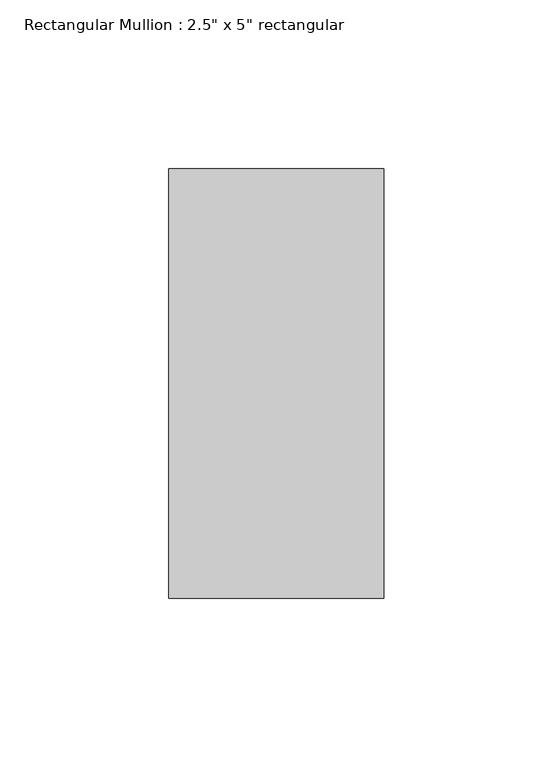
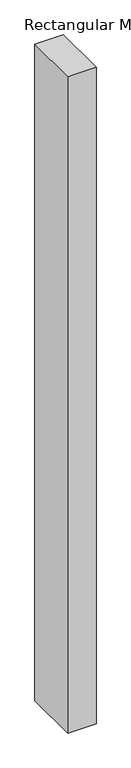
"""IFC4 building model written with IfcOpenShell, lengths in millimetres: member geometry."""

from ifc_helpers import new_model, si_unit, frame, origin, place, context, project, spatial, polyline, outline, extrude, source, transform, mapped, element, save


def member_ea390ee7(model_context):
    return source(origin(), model_context, "Body", "SweptSolid", [
        extrude(outline(polyline([(0.0, 63.5), (0.0, -63.5), (-63.5, -63.5), (-63.5, 63.5), (0.0, 63.5)])), frame((0.0, 0.0, -1551.6345763), z_axis=(0.0, 0.0, 1.0), x_axis=(1.0, 0.0, 0.0)), (0.0, 0.0, 1.0), 1551.6345763),
    ])


if __name__ == "__main__":
    model = new_model("IFC4")
    model_context = context("Model", 3, world=origin())
    ifc_project = project(units=[si_unit("LENGTHUNIT", "METRE", prefix="MILLI")], contexts=[model_context])
    site = spatial("IfcSite", under=ifc_project)
    building = spatial("IfcBuilding", under=site)
    placement = place(None, origin())
    member_shape = member_ea390ee7(model_context)
    element("IfcMember", 1, ObjectType="Rectangular Mullion : 2.5\" x 5\" rectangular", at=placement, inside=building, context=model_context, shape_type="MappedRepresentation", body=[
        mapped(member_shape, transform((0.0, 0.0, 0.0), x_axis=(1.0, 0.0, 0.0), y_axis=(0.0, 1.0, 0.0), z_axis=(0.0, 0.0, 1.0))),
    ])
    save(model, "model.ifc")

# Revit data of these elements
# Type "Rectangular Mullion : 2.5\" x 5\" rectangular"
#   built-in parameter 1007304 = 0.416667 (stored number, unit not read)
#   built-in parameter 1007301 = 0.104167 (stored number, unit not read)
#   built-in parameter 1007300 = 0.104167 (stored number, unit not read)
# Element 1 (IfcMember, "Rectangular Mullion : 2.5\" x 5\" rectangular")
#   Materials on its faces: "Aluminum"
# Materials
#   "Aluminum": class "Metal", colour RGB 247 247 247, transparency 0, Description = "Aluminum 6061", Cost = 0
